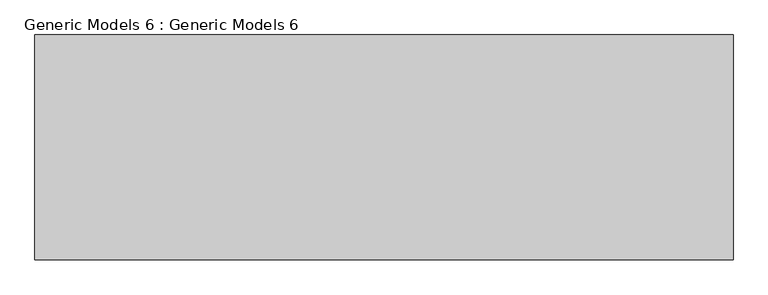
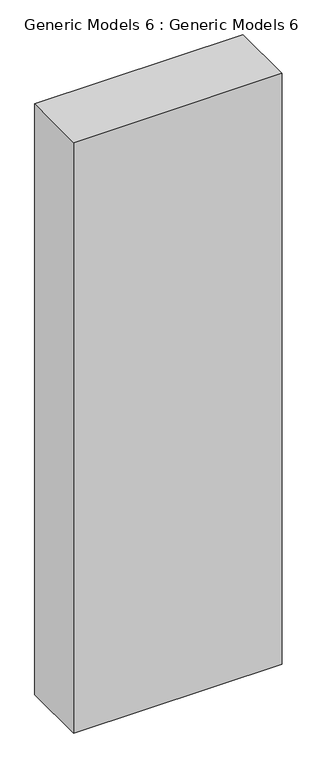
"""IFC4 building model written with IfcOpenShell, lengths in millimetres: proxy geometry, Generic Models 6 : Generic Models 6."""

from ifc_helpers import new_model, si_unit, origin, origin_with_axes, place, context, project, spatial, polyline, outline, extrude, source, transform, mapped, element, save


def generic_models_6_generic_models_6_789752cf(model_context):
    return source(origin(), model_context, "Body", "SweptSolid", [
        extrude(outline(polyline([(-3360.3120898, -8492.7980299), (-3360.3120898, -9178.5980299), (-5490.5493146, -9178.5980299), (-5490.5493146, -8492.7980299), (-3360.3120898, -8492.7980299)])), origin_with_axes(), (0.0, 0.0, 1.0), 6376.5429128),
    ])


if __name__ == "__main__":
    model = new_model("IFC4")
    model_context = context("Model", 3, world=origin())
    ifc_project = project(units=[si_unit("LENGTHUNIT", "METRE", prefix="MILLI")], contexts=[model_context])
    site = spatial("IfcSite", under=ifc_project)
    building = spatial("IfcBuilding", under=site)
    placement = place(None, origin())
    generic_models_6_generic_models_6_shape = generic_models_6_generic_models_6_789752cf(model_context)
    element("IfcBuildingElementProxy", 1, Name="Generic Models 6 : Generic Models 6", ObjectType="Generic Models 6 : Generic Models 6", at=placement, inside=building, context=model_context, shape_type="MappedRepresentation", body=[
        mapped(generic_models_6_generic_models_6_shape, transform((0.0, 0.0, 0.0), x_axis=(1.0, 0.0, 0.0), y_axis=(0.0, 1.0, 0.0), z_axis=(0.0, 0.0, 1.0))),
    ])
    save(model, "model.ifc")
